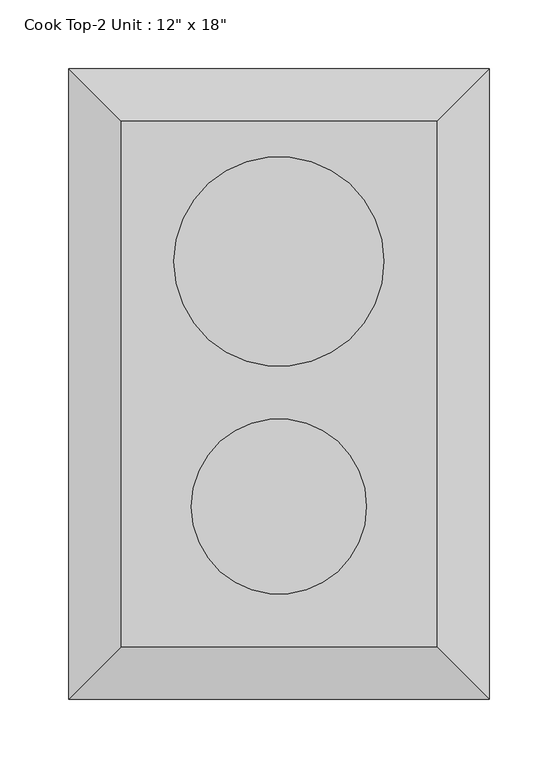
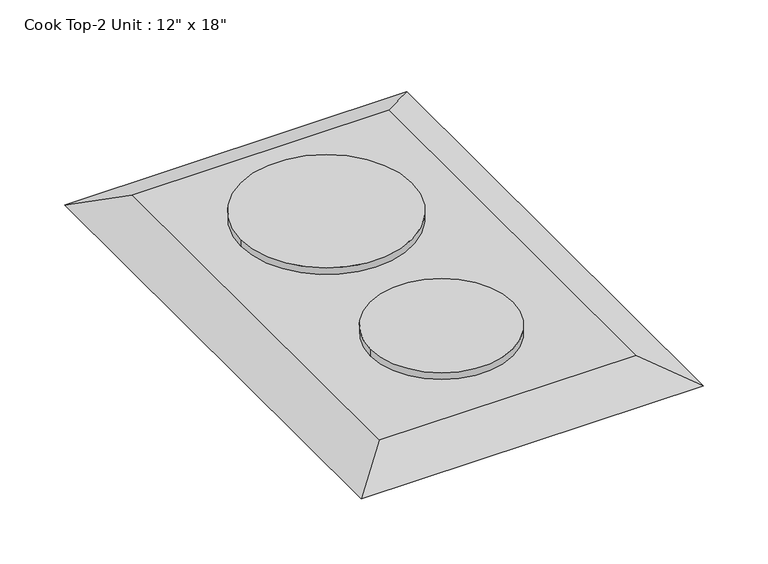
"""IFC4 building model written with IfcOpenShell, lengths in millimetres: proxy geometry."""

from ifc_helpers import new_model, si_unit, point, frame, frame_2d, origin, place, context, project, spatial, circle_curve, trimmed, segment, composite_curve, outline, extrude, faceted_brep, source, transform, mapped, element, save


def proxy_fe84b772(model_context):
    return source(origin(), model_context, "Body", "SolidModel", [
        extrude(outline(composite_curve([segment(trimmed(circle_curve(frame_2d((76.2, 119.1247956)), 76.2), [point((152.4, 119.1247956))], [point((0.0, 119.1247956))], False, "CARTESIAN"), True, "CONTINUOUS"), segment(trimmed(circle_curve(frame_2d((76.2, 119.1247956)), 76.2), [point((0.0, 119.1247956))], [point((152.4, 119.1247956))], False, "CARTESIAN"), True, "CONTINUOUS")], self_intersect=False)), frame((0.0, 0.0, 933.45), z_axis=(0.0, 0.0, 1.0), x_axis=(1.0, 0.0, 0.0)), (0.0, 0.0, 1.0), 6.35),
        extrude(outline(composite_curve([segment(trimmed(circle_curve(frame_2d((76.2, -58.6752044)), 63.5), [point((139.7, -58.6752044))], [point((12.7, -58.6752044))], False, "CARTESIAN"), True, "CONTINUOUS"), segment(trimmed(circle_curve(frame_2d((76.2, -58.6752044)), 63.5), [point((12.7, -58.6752044))], [point((139.7, -58.6752044))], False, "CARTESIAN"), True, "CONTINUOUS")], self_intersect=False)), frame((0.0, 0.0, 933.45), z_axis=(0.0, 0.0, 1.0), x_axis=(1.0, 0.0, 0.0)), (0.0, 0.0, 1.0), 6.35),
        faceted_brep([(190.5, 220.7247956, 933.45), (-38.1, 220.7247956, 933.45), (-38.1, -160.2752044, 933.45), (190.5, -160.2752044, 933.45), (228.6, 258.8247956, 914.4), (228.6, -198.3752044, 914.4), (-76.2, -198.3752044, 914.4), (-76.2, 258.8247956, 914.4)], [[[0, 1, 2, 3]], [[4, 5, 6, 7]], [[4, 7, 1, 0]], [[7, 6, 2, 1]], [[6, 5, 3, 2]], [[5, 4, 0, 3]]]),
    ])


if __name__ == "__main__":
    model = new_model("IFC4")
    model_context = context("Model", 3, world=origin())
    ifc_project = project(units=[si_unit("LENGTHUNIT", "METRE", prefix="MILLI")], contexts=[model_context])
    site = spatial("IfcSite", under=ifc_project)
    building = spatial("IfcBuilding", under=site)
    placement = place(None, origin())
    proxy_shape = proxy_fe84b772(model_context)
    element("IfcBuildingElementProxy", 1, Name="Cook Top-2 Unit : 12\" x 18\"", ObjectType="Cook Top-2 Unit : 12\" x 18\"", at=placement, inside=building, context=model_context, shape_type="MappedRepresentation", body=[
        mapped(proxy_shape, transform((0.0, 0.0, 0.0), x_axis=(1.0, 0.0, 0.0), y_axis=(0.0, 1.0, 0.0), z_axis=(0.0, 0.0, 1.0))),
    ])
    save(model, "model.ifc")

# Revit data of these elements
# Type "Cook Top-2 Unit : 12\" x 18\""
#   Assembly Code = "E1090400"
#   Counter Height = 3' - 0"
#   Depth = 1' - 6"
#   Width = 1' - 0"
#   Burner Material = Steel, Chrome Plated
#   Cooktop Material = Steel, Polished
#   Default Elevation = 0
# Element 1 (IfcBuildingElementProxy, "Cook Top-2 Unit : 12\" x 18\"")
#   Materials on its faces: "Steel, Chrome Plated", "Steel, Polished"
# Materials
#   "Steel, Chrome Plated": class "Metal", colour RGB 17 17 17, transparency 0, Description = "Chromiuim plated steel", Cost = 0
#   "Steel, Polished": class "Metal", colour RGB 57 57 57, transparency 0, Description = "Polished steel", Cost = 0
